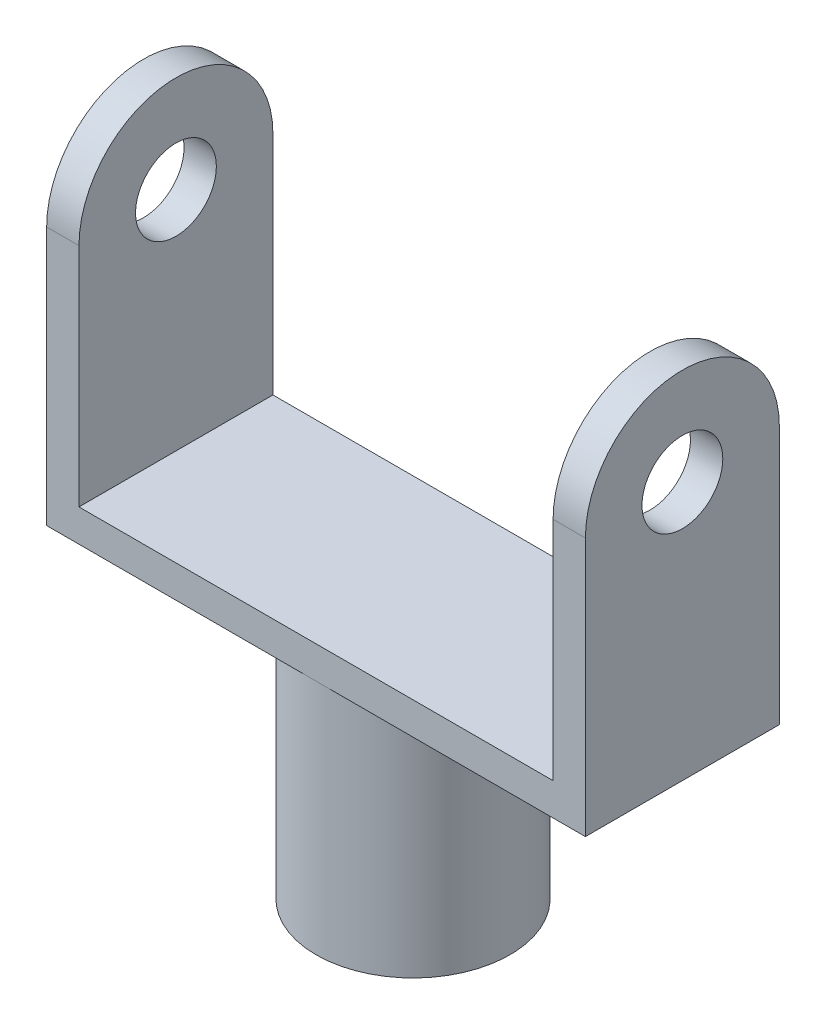
SolidWorks part; units mm, degrees
material "Plain Carbon Steel"
ref_plane "Front Plane" through (0, 0, 0) normal (0, 0, 1) x (1, 0, 0)
ref_plane "Top Plane" through (0, 0, 0) normal (0, 1, 0) x (1, 0, 0)
ref_plane "Right Plane" through (0, 0, 0) normal (1, 0, 0) x (0, 0, -1)
sketch "Stem Profile Ø36" plane through (0, 0, 0) normal (0, 1, 0) x (1, 0, 0)
  circle A0 centre (0, 0) radius 18
  dimension "D1" = 36
extrude "Stem Ø36x44" add sketch "Stem Profile Ø36" along normal blind 44
sketch "Base Plate Profile" plane through (0, 44, 0) normal (0, 1, 0) x (1, 0, 0)
  line L1 (-44, -18) -> (44, -18)
  line L2 (-44, -18) -> (-44, 18)
  line L3 (-44, 18) -> (44, 18)
  line L4 (44, -18) -> (44, 18)
  line L5 (-44, -18) -> (44, 18) construction
  line L6 (-44, 18) -> (44, -18) construction
  point P0 (0, 0)
  dimension "D1" = 36
  dimension "D2" = 88
extrude "Base Plate 88x36x6" add sketch "Base Plate Profile" along normal blind 6
sketch "Lug Profile with Pin Hole" plane through (44, 0, 0) normal (1, 0, 0) x (0, 0, -1)
  line L12 (-18, 44) -> (18, 44)
  line L13 (-18, 44) -> (-18, 92)
  line L15 (18, 44) -> (18, 92)
  arc A0 (-18, 92) -> (18, 92) centre (0, 92) cw
  circle A1 centre (0, 92) radius 7.5
  dimension "D3" = 15
  dimension "D1" = 18
  dimension "D2" = 48
  dimension "D4" = 36
extrude "Lug 6mm" add sketch "Lug Profile with Pin Hole" along normal blind 6
mirror "Lug Mirror" about plane through (0, 0, 0) normal (1, 0, 0) of "Lug 6mm"
